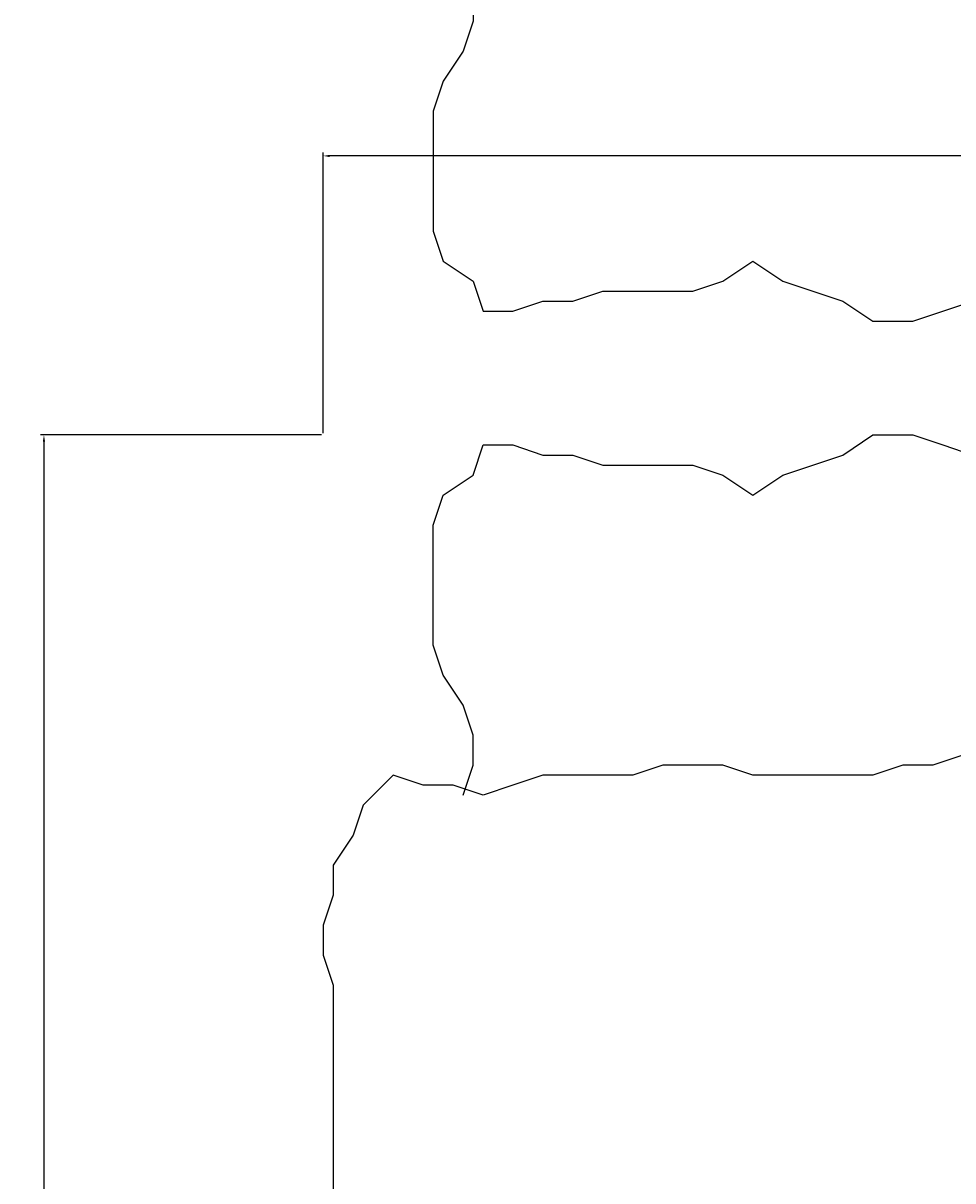
# Model space of a CAD drawing. Units: millimetres. Extents: x -857 to 54106, y -13666 to 13947.
# Tile 25 of 41: x 28665 to 29011, y 10747 to 11178. Entities that reach past the tile are written whole.
import ezdxf

# ---------------------------------------------------------------- set-up
doc = ezdxf.new("R2010")
doc.units = ezdxf.units.MM
doc.layers.add('A-ANNO-DIMS', color=2, linetype='Continuous', lineweight=18)
doc.layers.add('A-FURN', color=21, linetype='Continuous', lineweight=18)
doc.layers.add('TEFRIŞ', color=11, linetype='Continuous')
doc.styles.get("Standard").update_dxf_attribs({"font": 'arial.ttf'})
doc.dimstyles.new('ISO-25', dxfattribs={"dimtxt": 2.5, "dimasz": 2.5, "dimexe": 1.25, "dimexo": 0.625, "dimtad": 1, "dimtxsty": 'Standard', "dimcen": 2.5, "dimadec": 0, "dimazin": 0, "dimtfac": 1, "dimtmove": 0, "dimatfit": 3, "dimfxl": 1, "dimarcsym": 0})

# ---------------------------------------------------------------- blocks, each defined once
blk = doc.blocks.new('25')
at = {"layer": 'TEFRIŞ'}
for p, q in [((-1892.583, -362.165), (-1892.583, -344.935)), ((-1892.091, -363.642), (-1892.583, -362.165)), ((-1892.091, -365.119), (-1892.091, -363.642)), ((-1892.583, -366.596), (-1892.091, -365.119)), ((-1892.583, -368.072), (-1892.583, -366.596)), ((-1893.567, -369.549), (-1892.583, -368.072)), ((-1894.059, -371.026), (-1893.567, -369.549)), ((-1895.535, -372.503), (-1894.059, -371.026)), ((-1902.914, -372.503), (-1901.438, -372.011)), ((-1901.438, -372.011), (-1899.963, -371.518)), ((-1899.963, -371.518), (-1898.487, -372.011)), ((-1898.979, -371.518), (-1899.471, -372.995)), ((-1898.487, -372.011), (-1897.011, -372.011)), ((-1897.011, -372.011), (-1895.535, -372.503)), ((-1920.625, -372.995), (-1919.149, -372.503)), ((-1919.149, -372.503), (-1913.245, -372.503)), ((-1913.245, -372.503), (-1911.769, -372.995)), ((-1908.818, -372.995), (-1907.342, -372.503)), ((-1907.342, -372.503), (-1902.914, -372.503)), ((-1923.576, -373.488), (-1922.101, -372.995)), ((-1922.101, -372.995), (-1920.625, -372.995)), ((-1911.769, -372.995), (-1908.818, -372.995)), ((-1899.471, -372.995), (-1899.471, -374.472)), ((-1899.471, -374.472), (-1898.979, -375.949)), ((-1898.979, -375.949), (-1897.995, -377.426)), ((-1897.995, -377.426), (-1897.503, -378.903)), ((-1897.503, -378.903), (-1897.503, -384.81)), ((-1897.503, -384.81), (-1897.995, -386.287)), ((-1913.245, -386.287), (-1914.721, -387.272)), ((-1911.769, -387.272), (-1913.245, -386.287)), ((-1897.995, -386.287), (-1899.471, -387.272)), ((-1914.721, -387.272), (-1916.197, -387.764)), ((-1910.294, -387.764), (-1911.769, -387.272)), ((-1899.471, -387.272), (-1899.963, -388.749)), ((-1916.197, -387.764), (-1917.673, -388.256)), ((-1905.866, -387.764), (-1910.294, -387.764)), ((-1904.39, -388.256), (-1905.866, -387.764)), ((-1922.592, -388.749), (-1924.068, -388.256)), ((-1917.673, -388.256), (-1919.149, -389.241)), ((-1902.914, -388.256), (-1904.39, -388.256)), ((-1901.438, -388.749), (-1902.914, -388.256)), ((-1921.117, -389.241), (-1922.592, -388.749)), ((-1899.963, -388.749), (-1901.438, -388.749)), ((-1919.149, -389.241), (-1921.117, -389.241))]:
    blk.add_line(p, q, dxfattribs=at)
blk = doc.blocks.new('*D49')
at = {"layer": 'A-ANNO-DIMS', "color": 0, "lineweight": -2, "transparency": 16777216}
for p, q in [((28776.01, 11024.79), (28671.56, 11024.79)), ((28672.81, 11022.29), (28672.81, 10335.12)), ((28776.01, 10332.62), (28671.56, 10332.62))]:
    blk.add_line(p, q, dxfattribs=at)
at = {"layer": 'A-ANNO-DIMS', "color": 0, "transparency": 16777216}
for points in [[(28672.39, 11022.29), (28673.22, 11022.29), (28672.81, 11024.79)], [(28672.39, 10335.12), (28673.22, 10335.12), (28672.81, 10332.62)]]:
    blk.add_solid(points, dxfattribs=at)
at = {"layer": 'Defpoints', "color": 0, "transparency": 16777216}
for p in [(28776.63, 11024.79), (28672.81, 10332.62), (28776.63, 10332.62)]:
    blk.add_point(p, dxfattribs=at)
at = {"layer": 'A-ANNO-DIMS', "color": 0, "transparency": 16777216, "insert": (28670.89, 10678.71), "char_height": 2.5, "attachment_point": 5, "rotation": 90}
blk.add_mtext('CHAIR 692 TYP.', dxfattribs=at)
blk = doc.blocks.new('*D50')
at = {"layer": 'A-ANNO-DIMS', "color": 0, "lineweight": -2, "transparency": 16777216}
for p, q in [((28776.63, 11025.41), (28776.63, 11129.86)), ((29360.48, 11025.41), (29360.48, 11129.86)), ((29357.98, 11128.61), (28779.13, 11128.61))]:
    blk.add_line(p, q, dxfattribs=at)
at = {"layer": 'A-ANNO-DIMS', "color": 0, "transparency": 16777216}
for points in [[(28779.13, 11129.03), (28779.13, 11128.19), (28776.63, 11128.61)], [(29357.98, 11129.03), (29357.98, 11128.19), (29360.48, 11128.61)]]:
    blk.add_solid(points, dxfattribs=at)
at = {"layer": 'Defpoints', "color": 0, "transparency": 16777216}
for p in [(28776.63, 11128.61), (28776.63, 11024.79), (29360.48, 11024.79)]:
    blk.add_point(p, dxfattribs=at)
at = {"layer": 'A-ANNO-DIMS', "color": 0, "transparency": 16777216, "insert": (29068.56, 11130.51), "char_height": 2.5, "attachment_point": 5}
blk.add_mtext('584 TYP.', dxfattribs=at)

msp = doc.modelspace()

# ---------------------------------------------------------------- block references
at = {"layer": 'A-FURN', "xscale": -7.559220362162901, "yscale": 7.559220362162901, "zscale": 7.559220362162901}
msp.add_blockref('25', (14473.896, 14009.447), dxfattribs=at)
at = {"layer": 'A-FURN', "xscale": 7.559220362162901, "yscale": 7.559220362162901, "zscale": 7.559220362162901, "rotation": 180}
msp.add_blockref('25', (14473.896, 8082.429), dxfattribs=at)

# ---------------------------------------------------------------- dimensions: what is measured, and where the dimension line sits
at = {"layer": 'A-ANNO-DIMS'}
for base, p1, p2, angle, text, picture, middle in [((28776.63, 11128.611), (29360.482, 11024.786), (28776.63, 11024.786), 180, '<> TYP.', '*D50', (29068.556, 11130.512)), ((28672.806, 10332.624), (28776.63, 11024.786), (28776.63, 10332.624), 270, 'CHAIR <> TYP.', '*D49', (28670.888, 10678.705))]:
    dim = msp.add_linear_dim(base=base, p1=p1, p2=p2, angle=angle, text=text, dimstyle='ISO-25', override={"dimdec": 0, "dimrnd": 0, "dimzin": 0, "dimlunit": 2}, dxfattribs=at)
    dim.commit()
    dim.dimension.update_dxf_attribs({"geometry": picture, "text_midpoint": middle})

doc.saveas('drawing.dxf')
